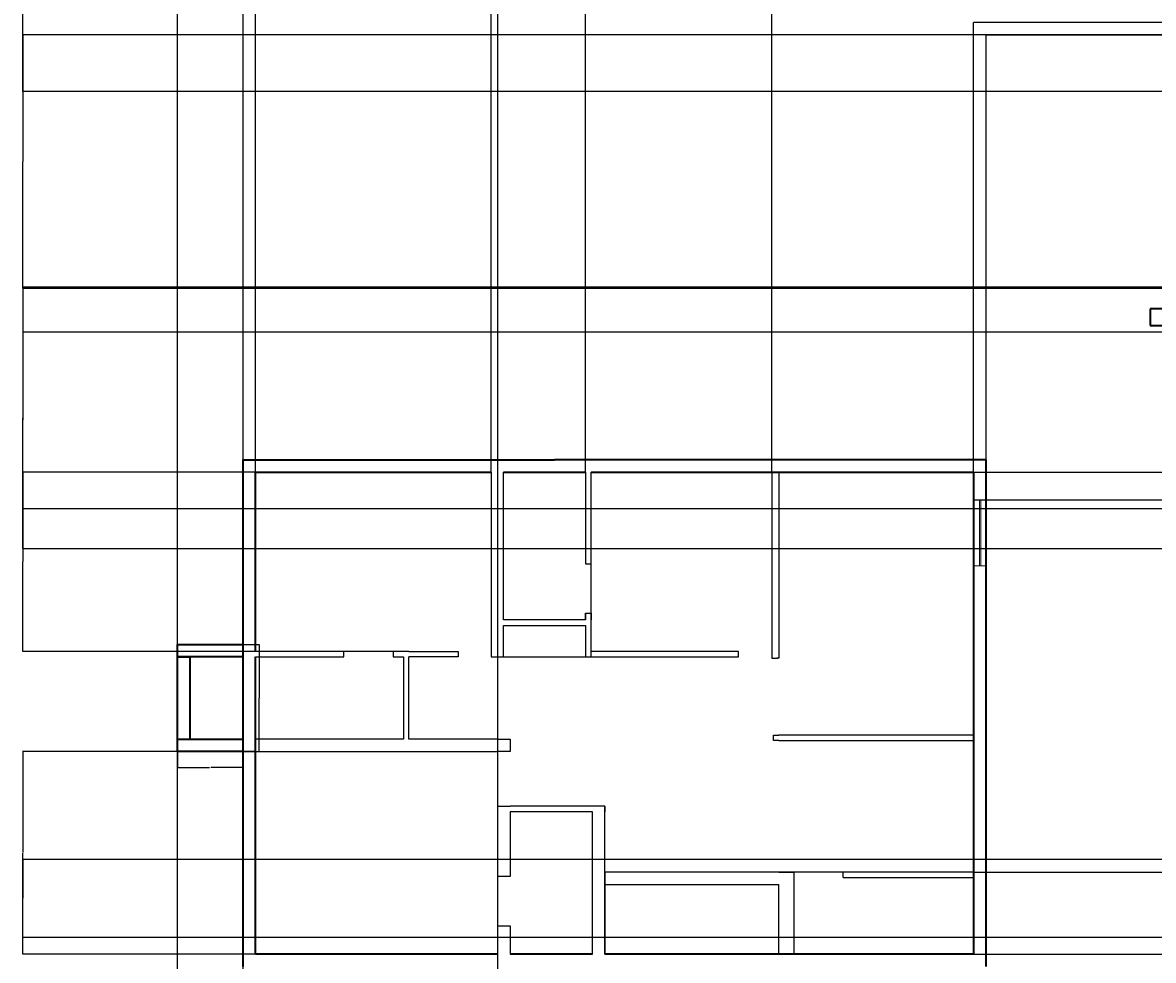
# Model space of a CAD drawing. Units: inches. Extents: x 2029 to 8798, y 1998 to 6373.
# Tile 2 of 11: x 2030 to 2855, y 4662 to 5347. Entities that reach past the tile are written whole.
import ezdxf

# ---------------------------------------------------------------- set-up
doc = ezdxf.new("R2010")
doc.units = ezdxf.units.IN
for name, color, linetype, lineweight in [('A-ANNO-DIMS', 2, 'Continuous', 18), ('A-GLAZ', 4, 'Continuous', 18), ('A-WALL-CIRC', 7, 'Continuous', 25), ('A-WALL-CORE', 7, 'Continuous', 35), ('A-WALL-EXTR', 7, 'Continuous', 35), ('A-WALL-INTR', 7, 'Continuous', 25)]:
    doc.layers.add(name, color=color, linetype=linetype, lineweight=lineweight)
doc.styles.get("Standard").update_dxf_attribs({"font": 'arial.ttf'})
doc.dimstyles.get("Standard").update_dxf_attribs({"dimtxt": 0.18, "dimasz": 0.18, "dimexe": 0.18, "dimexo": 0.0625, "dimgap": 0.09, "dimtad": 0, "dimtih": 1, "dimtoh": 1, "dimdec": 4, "dimzin": 0, "dimdsep": 46, "dimtxsty": 'Standard', "dimcen": 0.09, "dimadec": 0, "dimazin": 0, "dimtfac": 1, "dimtdec": 4, "dimtofl": 0, "dimtmove": 0, "dimatfit": 3, "dimfxl": 1, "dimtolj": 1, "dimtzin": 0, "dimarcsym": 0})

# ---------------------------------------------------------------- blocks, each defined once
blk = doc.blocks.new('WIN-48')
for p, q in [((0, 48), (9, 48)), ((4.5, 48), (4.5, 0)), ((5.5, 48), (5.5, 0)), ((9, 0), (0, 0))]:
    blk.add_line(p, q)
blk = doc.blocks.new('WALL-BAY-78X48')
for p, q in [((0, 69), (0, 78)), ((0, 78), (48, 78)), ((48, 69), (0, 69)), ((0, 9), (0, 69)), ((0, 69), (9, 69)), ((9, 69), (9, 9)), ((0, 0), (0, 9)), ((0, 9), (48, 9)), ((48, 0), (0, 0))]:
    blk.add_line(p, q)
blk = doc.blocks.new('*D35')
at = {"layer": 'A-ANNO-DIMS', "color": 0, "lineweight": -2, "transparency": 16777216}
for p, q in [((2190.6, 4892.96), (2202.42, 4892.96)), ((2202.24, 4892.78), (2202.24, 4854.14)), ((2202.24, 4815.14), (2202.24, 4853.78)), ((2190.6, 4814.96), (2202.42, 4814.96))]:
    blk.add_line(p, q, dxfattribs=at)
at = {"layer": 'A-ANNO-DIMS', "color": 0, "transparency": 16777216}
for points in [[(2202.21, 4892.78), (2202.27, 4892.78), (2202.24, 4892.96)], [(2202.21, 4815.14), (2202.27, 4815.14), (2202.24, 4814.96)]]:
    blk.add_solid(points, dxfattribs=at)
at = {"layer": 'Defpoints', "color": 0, "transparency": 16777216}
for p in [(2190.54, 4892.96), (2202.24, 4892.96), (2190.54, 4814.96)]:
    blk.add_point(p, dxfattribs=at)
at = {"layer": 'A-ANNO-DIMS', "color": 0, "transparency": 16777216, "insert": (2202.24, 4853.96), "char_height": 0.18, "attachment_point": 5}
blk.add_mtext('\\A1;WALL BAY 78 TYP.', dxfattribs=at)
blk = doc.blocks.new('*D36')
at = {"layer": 'A-ANNO-DIMS', "color": 0, "lineweight": -2, "transparency": 16777216}
for p, q in [((2142.54, 4814.9), (2142.54, 4803.08)), ((2190.54, 4814.9), (2190.54, 4803.08)), ((2142.72, 4803.26), (2166.01, 4803.26)), ((2190.36, 4803.26), (2167.07, 4803.26))]:
    blk.add_line(p, q, dxfattribs=at)
at = {"layer": 'A-ANNO-DIMS', "color": 0, "transparency": 16777216}
for points in [[(2142.72, 4803.29), (2142.72, 4803.23), (2142.54, 4803.26)], [(2190.36, 4803.29), (2190.36, 4803.23), (2190.54, 4803.26)]]:
    blk.add_solid(points, dxfattribs=at)
at = {"layer": 'Defpoints', "color": 0, "transparency": 16777216}
for p in [(2142.54, 4814.96), (2190.54, 4814.96), (2190.54, 4803.26)]:
    blk.add_point(p, dxfattribs=at)
at = {"layer": 'A-ANNO-DIMS', "color": 0, "transparency": 16777216, "insert": (2166.54, 4803.26), "char_height": 0.18, "attachment_point": 5}
blk.add_mtext('\\A1;48 TYP.', dxfattribs=at)
blk = doc.blocks.new('*D45')
at = {"layer": 'A-ANNO-DIMS', "color": 0, "lineweight": -2, "transparency": 16777216}
for p, q in [((2199.54, 5019.02), (2199.54, 6372.54)), ((2199.72, 6372.36), (2285.26, 6372.36)), ((2371.36, 6372.36), (2285.82, 6372.36)), ((2371.54, 5019.02), (2371.54, 6372.54))]:
    blk.add_line(p, q, dxfattribs=at)
at = {"layer": 'A-ANNO-DIMS', "color": 0, "transparency": 16777216}
for points in [[(2199.72, 6372.39), (2199.72, 6372.33), (2199.54, 6372.36)], [(2371.36, 6372.39), (2371.36, 6372.33), (2371.54, 6372.36)]]:
    blk.add_solid(points, dxfattribs=at)
at = {"layer": 'Defpoints', "color": 0, "transparency": 16777216}
for p in [(2371.54, 6372.36), (2199.54, 5018.96), (2371.54, 5018.96)]:
    blk.add_point(p, dxfattribs=at)
at = {"layer": 'A-ANNO-DIMS', "color": 0, "transparency": 16777216, "insert": (2285.54, 6372.36), "char_height": 0.18, "attachment_point": 5}
blk.add_mtext('\\A1;172', dxfattribs=at)
blk = doc.blocks.new('*D46')
at = {"layer": 'A-ANNO-DIMS', "color": 0, "lineweight": -2, "transparency": 16777216}
for p, q in [((2371.54, 5019.02), (2371.54, 6372.54)), ((2371.72, 6372.36), (2405.82, 6372.36)), ((2440.36, 6372.36), (2406.26, 6372.36)), ((2440.54, 5019.02), (2440.54, 6372.54))]:
    blk.add_line(p, q, dxfattribs=at)
at = {"layer": 'A-ANNO-DIMS', "color": 0, "transparency": 16777216}
for points in [[(2371.72, 6372.39), (2371.72, 6372.33), (2371.54, 6372.36)], [(2440.36, 6372.39), (2440.36, 6372.33), (2440.54, 6372.36)]]:
    blk.add_solid(points, dxfattribs=at)
at = {"layer": 'Defpoints', "color": 0, "transparency": 16777216}
for p in [(2440.54, 6372.36), (2371.54, 5018.96), (2440.54, 5018.96)]:
    blk.add_point(p, dxfattribs=at)
at = {"layer": 'A-ANNO-DIMS', "color": 0, "transparency": 16777216, "insert": (2406.04, 6372.36), "char_height": 0.18, "attachment_point": 5}
blk.add_mtext('\\A1;69', dxfattribs=at)
blk = doc.blocks.new('*D47')
at = {"layer": 'A-ANNO-DIMS', "color": 0, "lineweight": -2, "transparency": 16777216}
for p, q in [((2440.54, 5019.02), (2440.54, 6372.54)), ((2440.72, 6372.36), (2508.26, 6372.36)), ((2576.36, 6372.36), (2508.82, 6372.36)), ((2576.54, 5019.02), (2576.54, 6372.54))]:
    blk.add_line(p, q, dxfattribs=at)
at = {"layer": 'A-ANNO-DIMS', "color": 0, "transparency": 16777216}
for points in [[(2440.72, 6372.39), (2440.72, 6372.33), (2440.54, 6372.36)], [(2576.36, 6372.39), (2576.36, 6372.33), (2576.54, 6372.36)]]:
    blk.add_solid(points, dxfattribs=at)
at = {"layer": 'Defpoints', "color": 0, "transparency": 16777216}
for p in [(2576.54, 6372.36), (2440.54, 5018.96), (2576.54, 5018.96)]:
    blk.add_point(p, dxfattribs=at)
at = {"layer": 'A-ANNO-DIMS', "color": 0, "transparency": 16777216, "insert": (2508.54, 6372.36), "char_height": 0.18, "attachment_point": 5}
blk.add_mtext('\\A1;136', dxfattribs=at)
blk = doc.blocks.new('*D48')
at = {"layer": 'A-ANNO-DIMS', "color": 0, "lineweight": -2, "transparency": 16777216}
for p, q in [((2199.48, 4814.96), (2029.61, 4814.96)), ((2029.79, 4814.78), (2029.79, 4741.14)), ((2029.79, 4667.14), (2029.79, 4740.78)), ((2199.48, 4666.96), (2029.61, 4666.96))]:
    blk.add_line(p, q, dxfattribs=at)
at = {"layer": 'A-ANNO-DIMS', "color": 0, "transparency": 16777216}
for points in [[(2029.76, 4814.78), (2029.82, 4814.78), (2029.79, 4814.96)], [(2029.76, 4667.14), (2029.82, 4667.14), (2029.79, 4666.96)]]:
    blk.add_solid(points, dxfattribs=at)
at = {"layer": 'Defpoints', "color": 0, "transparency": 16777216}
for p in [(2029.79, 4814.96), (2199.54, 4814.96), (2199.54, 4666.96)]:
    blk.add_point(p, dxfattribs=at)
at = {"layer": 'A-ANNO-DIMS', "color": 0, "transparency": 16777216, "insert": (2029.79, 4740.96), "char_height": 0.18, "attachment_point": 5}
blk.add_mtext('\\A1;148', dxfattribs=at)
blk = doc.blocks.new('*D49')
at = {"layer": 'A-ANNO-DIMS', "color": 0, "lineweight": -2, "transparency": 16777216}
for p, q in [((2190.54, 4210.05), (2190.54, 6372.54)), ((2190.72, 6372.36), (2283.26, 6372.36)), ((2376.36, 6372.36), (2283.82, 6372.36)), ((2376.54, 4210.05), (2376.54, 6372.54))]:
    blk.add_line(p, q, dxfattribs=at)
at = {"layer": 'A-ANNO-DIMS', "color": 0, "transparency": 16777216}
for points in [[(2190.72, 6372.39), (2190.72, 6372.33), (2190.54, 6372.36)], [(2376.36, 6372.39), (2376.36, 6372.33), (2376.54, 6372.36)]]:
    blk.add_solid(points, dxfattribs=at)
at = {"layer": 'Defpoints', "color": 0, "transparency": 16777216}
for p in [(2376.54, 6372.36), (2190.54, 4209.99), (2376.54, 4209.99)]:
    blk.add_point(p, dxfattribs=at)
at = {"layer": 'A-ANNO-DIMS', "color": 0, "transparency": 16777216, "insert": (2283.54, 6372.36), "char_height": 0.18, "attachment_point": 5}
blk.add_mtext('\\A1;186', dxfattribs=at)
blk = doc.blocks.new('*D65')
at = {"layer": 'A-ANNO-DIMS', "color": 0, "lineweight": -2, "transparency": 16777216}
for p, q in [((3405.47, 5337.99), (2029.61, 5337.99)), ((2029.79, 5337.81), (2029.79, 5245.67)), ((2029.79, 5153.17), (2029.79, 5245.31)), ((3405.47, 5152.99), (2029.61, 5152.99))]:
    blk.add_line(p, q, dxfattribs=at)
at = {"layer": 'A-ANNO-DIMS', "color": 0, "transparency": 16777216}
for points in [[(2029.76, 5337.81), (2029.82, 5337.81), (2029.79, 5337.99)], [(2029.76, 5153.17), (2029.82, 5153.17), (2029.79, 5152.99)]]:
    blk.add_solid(points, dxfattribs=at)
at = {"layer": 'Defpoints', "color": 0, "transparency": 16777216}
for p in [(2029.79, 5337.99), (3405.53, 5337.99), (3405.53, 5152.99)]:
    blk.add_point(p, dxfattribs=at)
at = {"layer": 'A-ANNO-DIMS', "color": 0, "transparency": 16777216, "insert": (2029.79, 5245.49), "char_height": 0.18, "attachment_point": 5}
blk.add_mtext('\\A1;185', dxfattribs=at)
blk = doc.blocks.new('*D66')
at = {"layer": 'A-ANNO-DIMS', "color": 0, "lineweight": -2, "transparency": 16777216}
for p, q in [((2960.47, 5153.99), (2029.61, 5153.99)), ((2029.79, 5153.81), (2029.79, 5058.67)), ((2029.79, 4963.17), (2029.79, 5058.31)), ((2960.47, 4962.99), (2029.61, 4962.99))]:
    blk.add_line(p, q, dxfattribs=at)
at = {"layer": 'A-ANNO-DIMS', "color": 0, "transparency": 16777216}
for points in [[(2029.76, 5153.81), (2029.82, 5153.81), (2029.79, 5153.99)], [(2029.76, 4963.17), (2029.82, 4963.17), (2029.79, 4962.99)]]:
    blk.add_solid(points, dxfattribs=at)
at = {"layer": 'Defpoints', "color": 0, "transparency": 16777216}
for p in [(2029.79, 5153.99), (2960.53, 5153.99), (2960.53, 4962.99)]:
    blk.add_point(p, dxfattribs=at)
at = {"layer": 'A-ANNO-DIMS', "color": 0, "transparency": 16777216, "insert": (2029.79, 5058.49), "char_height": 0.18, "attachment_point": 5}
blk.add_mtext('\\A1;191', dxfattribs=at)
blk = doc.blocks.new('*D88')
at = {"layer": 'A-ANNO-DIMS', "color": 0, "lineweight": -2, "transparency": 16777216}
for p, q in [((2142.54, 4445.05), (2142.54, 6372.54)), ((2142.72, 6372.36), (3266.19, 6372.36)), ((4390.59, 6372.36), (3267.12, 6372.36)), ((4390.77, 4574.05), (4390.77, 6372.54))]:
    blk.add_line(p, q, dxfattribs=at)
at = {"layer": 'A-ANNO-DIMS', "color": 0, "transparency": 16777216}
for points in [[(2142.72, 6372.39), (2142.72, 6372.33), (2142.54, 6372.36)], [(4390.59, 6372.39), (4390.59, 6372.33), (4390.77, 6372.36)]]:
    blk.add_solid(points, dxfattribs=at)
at = {"layer": 'Defpoints', "color": 0, "transparency": 16777216}
for p in [(4390.77, 6372.36), (4390.77, 4573.99), (2142.54, 4444.99)]:
    blk.add_point(p, dxfattribs=at)
at = {"layer": 'A-ANNO-DIMS', "color": 0, "transparency": 16777216, "insert": (3266.65, 6372.36), "char_height": 0.18, "attachment_point": 5}
blk.add_mtext('\\A1;2248.2', dxfattribs=at)
blk = doc.blocks.new('*D91')
at = {"layer": 'A-ANNO-DIMS', "color": 0, "lineweight": -2, "transparency": 16777216}
for p, q in [((4095.32, 4736.09), (2029.61, 4736.09)), ((2029.79, 4735.91), (2029.79, 4707.78)), ((2029.79, 4679.27), (2029.79, 4707.41)), ((4095.32, 4679.09), (2029.61, 4679.09))]:
    blk.add_line(p, q, dxfattribs=at)
at = {"layer": 'A-ANNO-DIMS', "color": 0, "transparency": 16777216}
for points in [[(2029.76, 4735.91), (2029.82, 4735.91), (2029.79, 4736.09)], [(2029.76, 4679.27), (2029.82, 4679.27), (2029.79, 4679.09)]]:
    blk.add_solid(points, dxfattribs=at)
at = {"layer": 'Defpoints', "color": 0, "transparency": 16777216}
for p in [(2029.79, 4736.09), (4095.39, 4736.09), (4095.39, 4679.09)]:
    blk.add_point(p, dxfattribs=at)
at = {"layer": 'A-ANNO-DIMS', "color": 0, "transparency": 16777216, "insert": (2029.79, 4707.59), "char_height": 0.18, "attachment_point": 5}
blk.add_mtext('\\A1;57', dxfattribs=at)
blk = doc.blocks.new('*D105')
at = {"layer": 'A-ANNO-DIMS', "color": 0, "lineweight": -2, "transparency": 16777216}
for p, q in [((3968.7, 5479.61), (2029.61, 5479.61)), ((2029.79, 5479.43), (2029.79, 5388.29)), ((2029.79, 5296.79), (2029.79, 5387.93)), ((3968.7, 5296.61), (2029.61, 5296.61))]:
    blk.add_line(p, q, dxfattribs=at)
at = {"layer": 'A-ANNO-DIMS', "color": 0, "transparency": 16777216}
for points in [[(2029.76, 5479.43), (2029.82, 5479.43), (2029.79, 5479.61)], [(2029.76, 5296.79), (2029.82, 5296.79), (2029.79, 5296.61)]]:
    blk.add_solid(points, dxfattribs=at)
at = {"layer": 'Defpoints', "color": 0, "transparency": 16777216}
for p in [(2029.79, 5479.61), (3968.77, 5479.61), (3968.77, 5296.61)]:
    blk.add_point(p, dxfattribs=at)
at = {"layer": 'A-ANNO-DIMS', "color": 0, "transparency": 16777216, "insert": (2029.79, 5388.11), "char_height": 0.18, "attachment_point": 5}
blk.add_mtext('\\A1;183', dxfattribs=at)
blk = doc.blocks.new('*D106')
at = {"layer": 'A-ANNO-DIMS', "color": 0, "lineweight": -2, "transparency": 16777216}
for p, q in [((4325.32, 5121.09), (2029.61, 5121.09)), ((2029.79, 5120.91), (2029.79, 5056.78)), ((2029.79, 4992.27), (2029.79, 5056.41)), ((4325.32, 4992.09), (2029.61, 4992.09))]:
    blk.add_line(p, q, dxfattribs=at)
at = {"layer": 'A-ANNO-DIMS', "color": 0, "transparency": 16777216}
for points in [[(2029.76, 5120.91), (2029.82, 5120.91), (2029.79, 5121.09)], [(2029.76, 4992.27), (2029.82, 4992.27), (2029.79, 4992.09)]]:
    blk.add_solid(points, dxfattribs=at)
at = {"layer": 'Defpoints', "color": 0, "transparency": 16777216}
for p in [(4325.39, 5121.09), (2029.79, 4992.09), (4325.39, 4992.09)]:
    blk.add_point(p, dxfattribs=at)
at = {"layer": 'A-ANNO-DIMS', "color": 0, "transparency": 16777216, "insert": (2029.79, 5056.59), "char_height": 0.18, "attachment_point": 5}
blk.add_mtext('\\A1;129', dxfattribs=at)
blk = doc.blocks.new('*D110')
at = {"layer": 'A-ANNO-DIMS', "color": 0, "lineweight": -2, "transparency": 16777216}
for p, q in [((2723.6, 5018.96), (4503.7, 5018.96)), ((4503.52, 5018.78), (4503.52, 5008.93)), ((4503.52, 4998.71), (4503.52, 5008.56)), ((2723.6, 4998.53), (4503.7, 4998.53))]:
    blk.add_line(p, q, dxfattribs=at)
at = {"layer": 'A-ANNO-DIMS', "color": 0, "transparency": 16777216}
for points in [[(4503.49, 5018.78), (4503.55, 5018.78), (4503.52, 5018.96)], [(4503.49, 4998.71), (4503.55, 4998.71), (4503.52, 4998.53)]]:
    blk.add_solid(points, dxfattribs=at)
at = {"layer": 'Defpoints', "color": 0, "transparency": 16777216}
for p in [(2723.54, 5018.96), (2723.54, 4998.53), (4503.52, 4998.53)]:
    blk.add_point(p, dxfattribs=at)
at = {"layer": 'A-ANNO-DIMS', "color": 0, "transparency": 16777216, "insert": (4503.52, 5008.75), "char_height": 0.18, "attachment_point": 5}
blk.add_mtext('\\A1;20.425', dxfattribs=at)
blk = doc.blocks.new('*D111')
at = {"layer": 'A-ANNO-DIMS', "color": 0, "lineweight": -2, "transparency": 16777216}
for p, q in [((2723.6, 4726.96), (4503.7, 4726.96)), ((4503.52, 4726.78), (4503.52, 4697.16)), ((4503.52, 4667.17), (4503.52, 4696.79)), ((2723.6, 4666.99), (4503.7, 4666.99))]:
    blk.add_line(p, q, dxfattribs=at)
at = {"layer": 'A-ANNO-DIMS', "color": 0, "transparency": 16777216}
for points in [[(4503.49, 4726.78), (4503.55, 4726.78), (4503.52, 4726.96)], [(4503.49, 4667.17), (4503.55, 4667.17), (4503.52, 4666.99)]]:
    blk.add_solid(points, dxfattribs=at)
at = {"layer": 'Defpoints', "color": 0, "transparency": 16777216}
for p in [(2723.54, 4726.96), (4503.52, 4726.96), (2723.54, 4666.99)]:
    blk.add_point(p, dxfattribs=at)
at = {"layer": 'A-ANNO-DIMS', "color": 0, "transparency": 16777216, "insert": (4503.52, 4696.97), "char_height": 0.18, "attachment_point": 5}
blk.add_mtext('\\A1;59.97', dxfattribs=at)
blk = doc.blocks.new('*D112')
at = {"layer": 'A-ANNO-DIMS', "color": 0, "lineweight": -2, "transparency": 16777216}
for p, q in [((2199.48, 5018.96), (2029.61, 5018.96)), ((2029.79, 5018.78), (2029.79, 4953.64)), ((2029.79, 4888.14), (2029.79, 4953.28)), ((2199.48, 4887.96), (2029.61, 4887.96))]:
    blk.add_line(p, q, dxfattribs=at)
at = {"layer": 'A-ANNO-DIMS', "color": 0, "transparency": 16777216}
for points in [[(2029.76, 5018.78), (2029.82, 5018.78), (2029.79, 5018.96)], [(2029.76, 4888.14), (2029.82, 4888.14), (2029.79, 4887.96)]]:
    blk.add_solid(points, dxfattribs=at)
at = {"layer": 'Defpoints', "color": 0, "transparency": 16777216}
for p in [(2029.79, 5018.96), (2199.54, 5018.96), (2199.54, 4887.96)]:
    blk.add_point(p, dxfattribs=at)
at = {"layer": 'A-ANNO-DIMS', "color": 0, "transparency": 16777216, "insert": (2029.79, 4953.46), "char_height": 0.18, "attachment_point": 5}
blk.add_mtext('\\A1;131', dxfattribs=at)

msp = doc.modelspace()

# ---------------------------------------------------------------- linework, layer by layer
at = {"layer": 'A-WALL-CIRC'}
for p, q in [((2723.5398, 5018.9585), (2723.5398, 5346.9886)), ((2732.5398, 5346.9886), (2723.5398, 5346.9886)), ((2951.5292, 5346.9886), (2732.5398, 5346.9886)), ((2732.5398, 5337.9886), (2951.5292, 5337.9886)), ((2732.5398, 5337.9886), (2732.5398, 5027.9585))]:
    msp.add_line(p, q, dxfattribs=at)
at = {"layer": 'A-WALL-CORE'}
for p, q in [((2864.5292, 5137.9886), (2852.5292, 5137.9886)), ((2852.5292, 5137.9886), (2852.5292, 5125.9886)), ((2852.5292, 5125.9886), (2951.5292, 5125.9886))]:
    msp.add_line(p, q, dxfattribs=at)
at = {"layer": 'A-WALL-EXTR'}
for p, q in [((2190.5398, 4657.9585), (2190.5398, 5027.9585)), ((2190.5398, 5027.9585), (2401.3042, 5027.9585)), ((2401.3042, 5027.9585), (2417.7365, 5027.9585)), ((2732.5398, 5027.9585), (2417.7365, 5027.9585)), ((2732.5398, 5027.9585), (2732.5398, 4666.9886)), ((2199.5398, 4887.9585), (2199.5398, 5018.9585)), ((2199.5398, 5018.9585), (2371.5398, 5018.9585)), ((2199.5398, 5018.9585), (2371.5398, 5018.9585)), ((2380.5398, 5018.9585), (2440.5398, 5018.9585)), ((2380.5398, 5018.9585), (2440.5398, 5018.9585)), ((2444.5398, 5018.9585), (2576.5398, 5018.9585)), ((2444.5398, 5018.9585), (2576.5398, 5018.9585)), ((2576.5398, 5018.9585), (2723.5398, 5018.9585)), ((2723.5398, 5018.9585), (2723.5398, 4998.5338)), ((2723.5398, 4998.5338), (2723.5398, 4948.7306)), ((2723.5398, 4950.5338), (2723.5398, 4666.9585)), ((2723.5398, 4950.5338), (2723.5398, 4826.9585)), ((2199.5398, 4666.9585), (2199.5398, 4883.9585)), ((2199.5398, 4823.9585), (2199.5398, 4883.9585)), ((2723.5398, 4822.9585), (2723.5398, 4726.9585)), ((2199.5398, 4666.9585), (2199.5398, 4814.9585)), ((2376.5398, 4666.9585), (2199.5398, 4666.9585)), ((2445.5398, 4666.9585), (2385.5398, 4666.9585)), ((2401.3042, 4666.9886), (2401.3042, 4666.9585)), ((2445.5398, 4666.9886), (2401.3042, 4666.9886)), ((2723.5398, 4666.9886), (2454.5398, 4666.9886)), ((2723.5398, 4666.9585), (2454.5398, 4666.9585)), ((2723.5398, 4666.9585), (2581.5398, 4666.9585)), ((2732.5398, 4666.9886), (2732.5398, 4657.9585))]:
    msp.add_line(p, q, dxfattribs=at)
at = {"layer": 'A-WALL-INTR'}
for p, q in [((2371.5398, 5018.9585), (2371.5398, 4883.9585)), ((2380.5398, 4910.9585), (2380.5398, 5018.9585)), ((2440.5398, 5018.9585), (2440.5398, 4951.957)), ((2444.5398, 4910.9585), (2444.5398, 5018.9585)), ((2576.5398, 5018.9585), (2576.5398, 4882.9585)), ((2581.5398, 5018.9585), (2581.5398, 4882.9585)), ((2440.5398, 4951.957), (2444.5398, 4951.957)), ((2440.5398, 4910.9585), (2380.5398, 4910.9585)), ((2440.5398, 4915.957), (2440.5398, 4910.9585)), ((2440.5398, 4910.9585), (2440.5398, 4915.957)), ((2440.5398, 4915.957), (2444.5398, 4915.957)), ((2444.5398, 4915.957), (2444.5398, 4910.9585)), ((2444.5398, 4906.9585), (2444.5398, 4910.9585)), ((2380.5398, 4883.9585), (2380.5398, 4906.9585)), ((2380.5398, 4906.9585), (2440.4529, 4906.9585)), ((2440.4529, 4906.9585), (2440.4529, 4883.9585)), ((2444.5398, 4883.9585), (2444.5398, 4906.9585)), ((2307.5398, 4887.9585), (2199.5398, 4887.9585)), ((2264.03, 4883.9585), (2264.03, 4887.9585)), ((2307.5398, 4887.9585), (2300.03, 4887.9585)), ((2300.03, 4887.9585), (2300.03, 4883.9585)), ((2311.5398, 4887.9585), (2307.5398, 4887.9585)), ((2311.5398, 4887.9585), (2347.5398, 4887.9585)), ((2347.5398, 4887.9585), (2347.5398, 4883.9585)), ((2552.1143, 4887.9585), (2444.5398, 4887.9585)), ((2552.1143, 4883.9585), (2552.1143, 4887.9585)), ((2199.5398, 4883.9585), (2264.03, 4883.9585)), ((2300.03, 4883.9585), (2307.5398, 4883.9585)), ((2307.5398, 4883.9585), (2307.5398, 4823.9585)), ((2311.5398, 4823.9585), (2311.5398, 4883.9585)), ((2347.5398, 4883.9585), (2311.5398, 4883.9585)), ((2371.5398, 4883.9585), (2380.5398, 4883.9585)), ((2380.5398, 4883.9585), (2444.5398, 4883.9585)), ((2440.4529, 4883.9585), (2444.5398, 4883.9585)), ((2444.5398, 4883.9585), (2552.1143, 4883.9585)), ((2576.5398, 4882.9585), (2580.5398, 4882.9585)), ((2581.5398, 4882.9585), (2579.9704, 4882.9585)), ((2307.5398, 4823.9585), (2199.5398, 4823.9585)), ((2376.5398, 4823.9585), (2311.5398, 4823.9585)), ((2376.5398, 4823.9585), (2385.5398, 4823.9585)), ((2385.5398, 4823.9585), (2385.5398, 4814.9585)), ((2577.5398, 4822.9585), (2577.5398, 4826.9585)), ((2577.5398, 4826.9585), (2581.5398, 4826.9585)), ((2581.5398, 4822.9585), (2577.5398, 4822.9585)), ((2723.5398, 4826.9585), (2581.5398, 4826.9585)), ((2581.5398, 4822.9585), (2723.5398, 4822.9585)), ((2199.5398, 4814.9585), (2376.5398, 4814.9585)), ((2385.5398, 4814.9585), (2376.5398, 4814.9585)), ((2376.5398, 4666.9585), (2376.5398, 4774.9585)), ((2376.5398, 4774.9585), (2385.5398, 4774.9585)), ((2445.5398, 4774.9585), (2385.5398, 4774.9585)), ((2385.5398, 4770.9585), (2385.5398, 4723.6299)), ((2445.5398, 4770.9585), (2385.5398, 4770.9585)), ((2454.5398, 4774.9585), (2445.5398, 4774.9585)), ((2445.5398, 4666.9585), (2445.5398, 4770.9585)), ((2454.5398, 4726.9585), (2454.5398, 4774.9585)), ((2454.5398, 4774.9585), (2454.5398, 4770.9585)), ((2385.5398, 4723.6299), (2376.5398, 4723.6299)), ((2445.5398, 4666.9585), (2445.5398, 4726.9585)), ((2454.5398, 4666.9585), (2454.5398, 4727.9585)), ((2581.5398, 4726.9585), (2454.5398, 4726.9585)), ((2454.5398, 4726.9585), (2454.5398, 4666.9585)), ((2454.5398, 4726.9585), (2454.5398, 4717.9585)), ((2723.5398, 4726.9585), (2581.5398, 4726.9585)), ((2581.5398, 4726.9585), (2592.544, 4726.9585)), ((2592.544, 4726.9585), (2592.544, 4722.9585)), ((2592.544, 4722.9585), (2592.544, 4666.9886)), ((2628.544, 4722.9585), (2628.544, 4726.9585)), ((2628.544, 4722.9585), (2723.5398, 4722.9585)), ((2454.5398, 4717.9585), (2581.5398, 4717.9585)), ((2581.5398, 4666.9585), (2581.5398, 4717.9585)), ((2376.5398, 4666.9585), (2376.5398, 4687.6299)), ((2376.5398, 4687.6299), (2385.5398, 4687.6299)), ((2385.5398, 4687.6299), (2385.5398, 4666.9585))]:
    msp.add_line(p, q, dxfattribs=at)

# ---------------------------------------------------------------- block references
at = {"layer": 'A-GLAZ'}
msp.add_blockref('WIN-48', (2723.5398, 4950.5338), dxfattribs=at)
at = {"layer": 'A-WALL-EXTR'}
msp.add_blockref('WALL-BAY-78X48', (2142.5398, 4814.9585), dxfattribs=at)

# ---------------------------------------------------------------- dimensions: what is measured, and where the dimension line sits
at = {"layer": 'A-ANNO-DIMS'}
for base, p1, p2, override, picture, middle in [((4390.7657, 6372.3623), (2142.5398, 4444.9886), (4390.7657, 4573.9886), {"dimdec": 1, "dimlfac": 1, "dimrnd": 0, "dimzin": 0, "dimdsep": 46, "dimlunit": 2}, '*D88', (3266.6528, 6372.3623)), ((2376.5398, 6372.3623), (2190.5398, 4209.9886), (2376.5398, 4209.9886), {"dimdec": 0, "dimlfac": 1, "dimrnd": 0, "dimzin": 0, "dimdsep": 46, "dimlunit": 2}, '*D49', (2283.5398, 6372.3623)), ((2371.5398, 6372.3623), (2199.5398, 5018.9585), (2371.5398, 5018.9585), {"dimdec": 0, "dimlfac": 1, "dimrnd": 0, "dimzin": 0, "dimdsep": 46, "dimlunit": 2}, '*D45', (2285.5398, 6372.3623)), ((2440.5398, 6372.3623), (2371.5398, 5018.9585), (2440.5398, 5018.9585), {"dimdec": 0, "dimlfac": 1, "dimrnd": 0, "dimzin": 0, "dimdsep": 46, "dimlunit": 2}, '*D46', (2406.0398, 6372.3623)), ((2576.5398, 6372.3623), (2440.5398, 5018.9585), (2576.5398, 5018.9585), {"dimdec": 0, "dimlfac": 1, "dimrnd": 0, "dimzin": 0, "dimdsep": 46, "dimlunit": 2}, '*D47', (2508.5398, 6372.3623))]:
    dim = msp.add_linear_dim(base=base, p1=p1, p2=p2, dimstyle='Standard', override=override, dxfattribs=at)
    dim.commit()
    dim.dimension.update_dxf_attribs({"geometry": picture, "text_midpoint": middle})
for base, p1, p2, override, picture, middle in [((2029.7898, 5479.6123), (3968.7657, 5296.6123), (3968.7657, 5479.6123), {"dimdec": 0, "dimlfac": 1, "dimrnd": 0, "dimzin": 0, "dimdsep": 46, "dimlunit": 2}, '*D105', (2029.7898, 5388.1123)), ((2029.7898, 5337.9886), (3405.5292, 5152.9886), (3405.5292, 5337.9886), {"dimdec": 0, "dimlfac": 1, "dimrnd": 0, "dimzin": 0, "dimdsep": 46, "dimlunit": 2}, '*D65', (2029.7898, 5245.4886)), ((2029.7898, 5153.9886), (2960.5292, 4962.9886), (2960.5292, 5153.9886), {"dimdec": 0, "dimlfac": 1, "dimrnd": 0, "dimzin": 0, "dimdsep": 46, "dimlunit": 2}, '*D66', (2029.7898, 5058.4886)), ((2029.7898, 4992.0948), (4325.3869, 5121.0948), (4325.3869, 4992.0948), {"dimdec": 0, "dimlfac": 1, "dimrnd": 0, "dimzin": 0, "dimdsep": 46, "dimlunit": 2}, '*D106', (2029.7898, 5056.5948)), ((2029.7898, 5018.9585), (2199.5398, 4887.9585), (2199.5398, 5018.9585), {"dimdec": 0, "dimlfac": 1, "dimrnd": 0, "dimzin": 0, "dimdsep": 46, "dimlunit": 2}, '*D112', (2029.7898, 4953.4585)), ((4503.5157, 4998.5338), (2723.5398, 5018.9585), (2723.5398, 4998.5338), {"dimdec": 3, "dimlfac": 1, "dimrnd": 0, "dimzin": 0, "dimdsep": 46, "dimlunit": 2}, '*D110', (4503.5157, 5008.7461)), ((2029.7898, 4814.9585), (2199.5398, 4666.9585), (2199.5398, 4814.9585), {"dimdec": 0, "dimlfac": 1, "dimrnd": 0, "dimzin": 0, "dimdsep": 46, "dimlunit": 2}, '*D48', (2029.7898, 4740.9585)), ((2029.7898, 4736.0948), (4095.3869, 4679.0948), (4095.3869, 4736.0948), {"dimdec": 0, "dimlfac": 1, "dimrnd": 0, "dimzin": 0, "dimdsep": 46, "dimlunit": 2}, '*D91', (2029.7898, 4707.5948)), ((4503.5157, 4726.9585), (2723.5398, 4666.9886), (2723.5398, 4726.9585), {"dimdec": 2, "dimlfac": 1, "dimrnd": 0, "dimzin": 0, "dimdsep": 46, "dimlunit": 2}, '*D111', (4503.5157, 4696.9735))]:
    dim = msp.add_linear_dim(base=base, p1=p1, p2=p2, angle=90, dimstyle='Standard', override=override, dxfattribs=at)
    dim.commit()
    dim.dimension.update_dxf_attribs({"geometry": picture, "text_midpoint": middle})
dim = msp.add_linear_dim(base=(2202.2398, 4892.9585), p1=(2190.5398, 4814.9585), p2=(2190.5398, 4892.9585), angle=90, text='WALL BAY <> TYP.', dimstyle='Standard', override={"dimdec": 0, "dimlfac": 1, "dimrnd": 0, "dimzin": 0, "dimdsep": 46, "dimlunit": 2}, dxfattribs=at)
dim.commit()
dim.dimension.update_dxf_attribs({"geometry": '*D35', "text_midpoint": (2202.2398, 4853.9585)})
dim = msp.add_linear_dim(base=(2190.5398, 4803.2585), p1=(2142.5398, 4814.9585), p2=(2190.5398, 4814.9585), text='<> TYP.', dimstyle='Standard', override={"dimdec": 0, "dimlfac": 1, "dimrnd": 0, "dimzin": 0, "dimdsep": 46, "dimlunit": 2}, dxfattribs=at)
dim.commit()
dim.dimension.update_dxf_attribs({"geometry": '*D36', "text_midpoint": (2166.5398, 4803.2585)})

doc.saveas('drawing.dxf')
